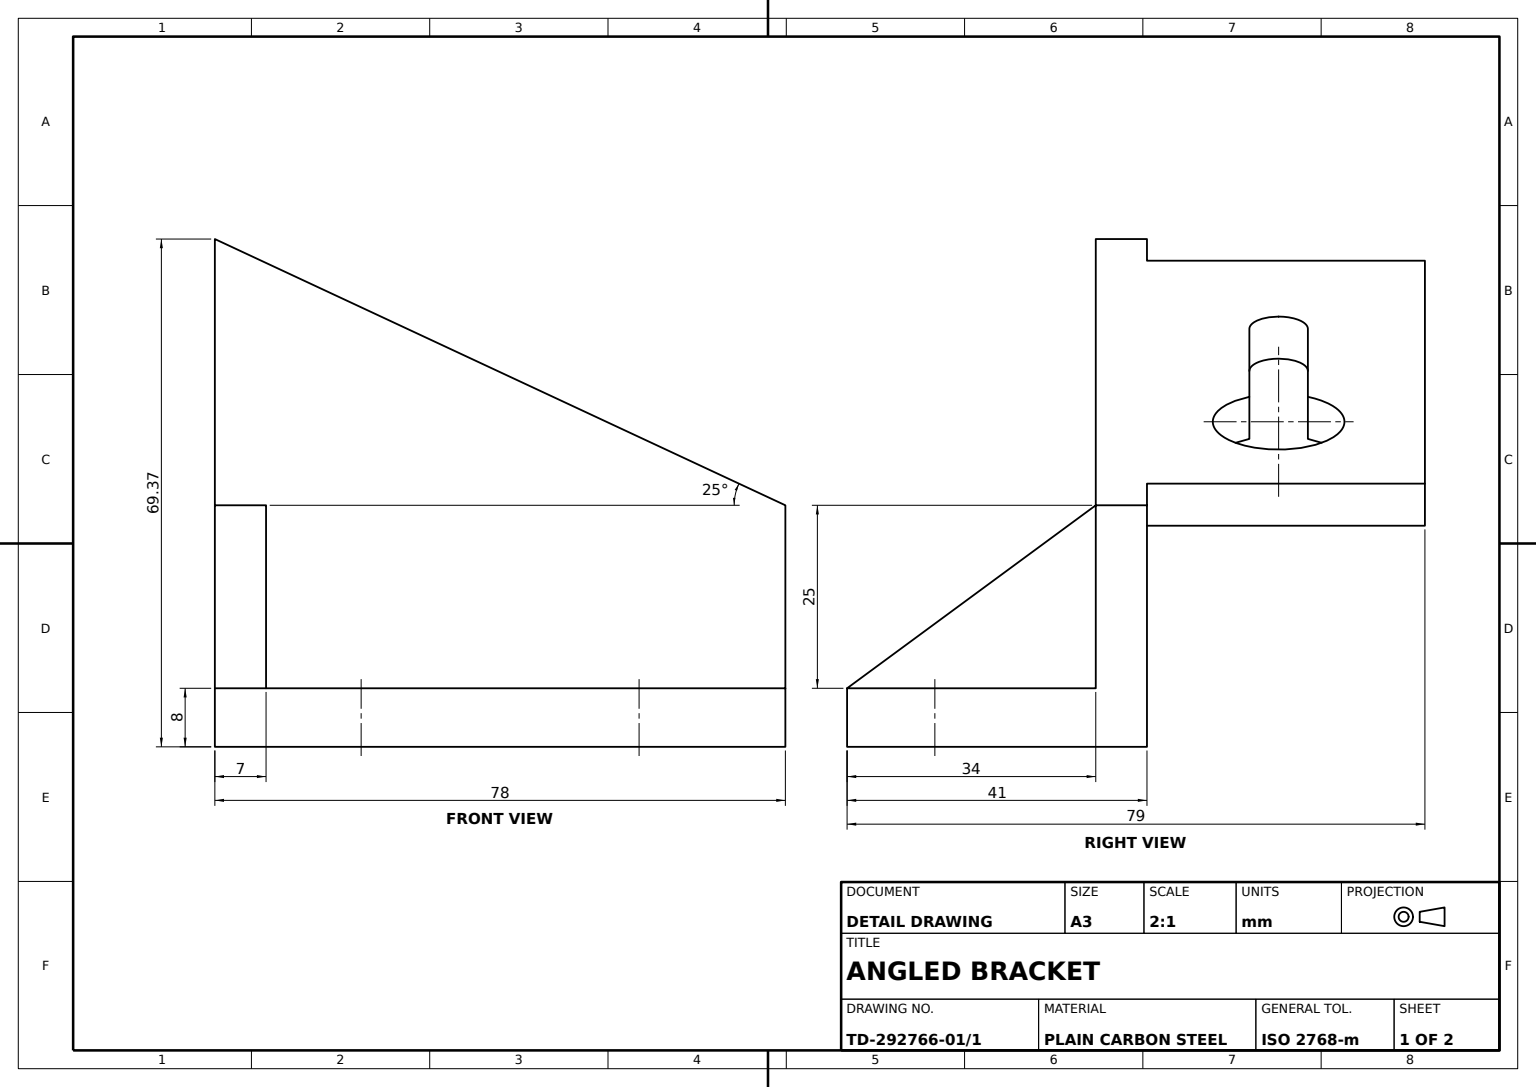
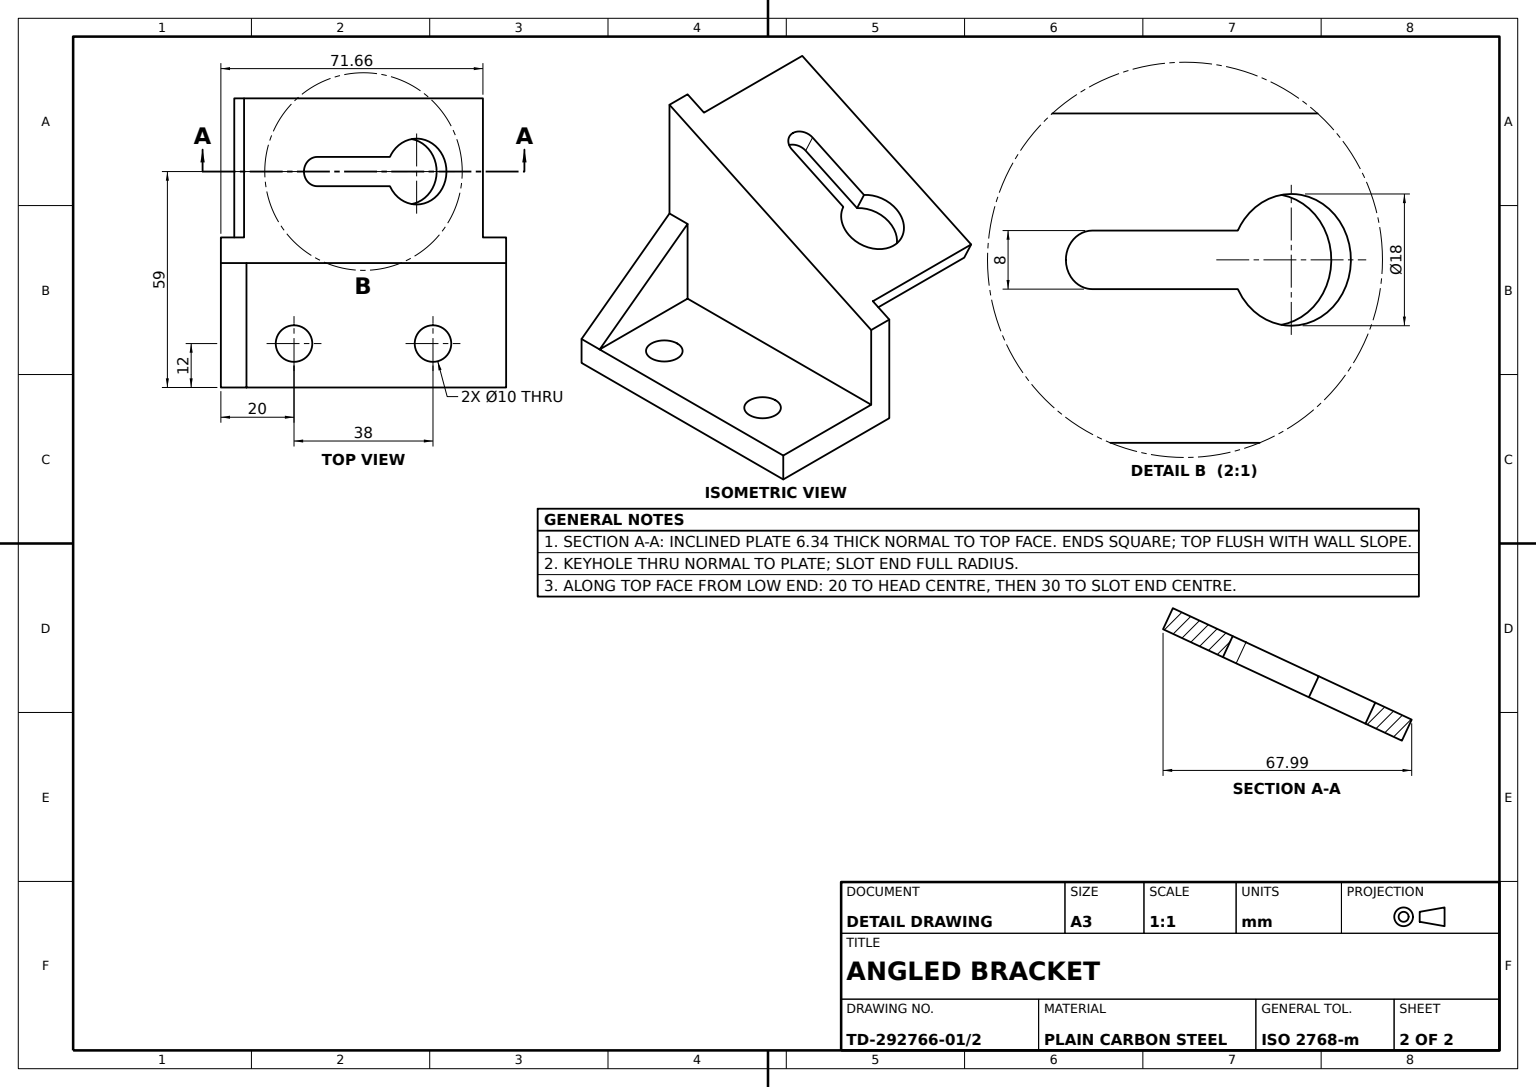
SolidWorks part; units mm, degrees
material "Plain Carbon Steel"
ref_plane "Front Plane" through (0, 0, 0) normal (0, 0, 1) x (1, 0, 0)
ref_plane "Top Plane" through (0, 0, 0) normal (0, 1, 0) x (1, 0, 0)
ref_plane "Right Plane" through (0, 0, 0) normal (1, 0, 0) x (0, 0, -1)
sketch "Base Plate Sketch" plane through (0, 0, 0) normal (0, 1, 0) x (1, 0, 0)
  line L1 (-39, -24.5) -> (39, -24.5)
  line L2 (-39, -24.5) -> (-39, 16.5)
  line L3 (-39, 16.5) -> (39, 16.5)
  line L4 (39, -24.5) -> (39, 16.5)
  circle A0 centre (-19, -12.5) radius 5
  circle A1 centre (19, -12.5) radius 5
  point P0 (0, 0)
  dimension "D3" = 10
  dimension "D4" = 10
  dimension "D1" = 78
  dimension "D2" = 41
  dimension "D5" = 12
  dimension "D6" = 20
  dimension "D7" = 20
  dimension "D8" = 12
  dimension "D9" = 39
  dimension "D10" = 24.5
extrude "Base Plate with Mounting Holes" add sketch "Base Plate Sketch" along normal blind 8
sketch "Upright Wall Sketch" plane through (0, 8, 0) normal (0, 1, 0) x (1, 0, 0)
  line L0 (-39, -24.5) -> (39, -24.5) construction
  line L1 (-39, 16.5) -> (-32, 16.5)
  line L2 (-39, 16.5) -> (-39, -24.5)
  line L3 (-39, -24.5) -> (-32, -24.5)
  line L4 (-32, 16.5) -> (-32, -24.5)
  dimension "D1" = 7
extrude "Upright Wall" add sketch "Upright Wall Sketch" along normal blind 38 contours L2 L3 L4 L1
sketch "Back Plate Sketch" plane through (0, 8, 0) normal (0, 1, 0) x (1, 0, 0)
  line L0 (39, -24.5) -> (39, 16.5) construction
  line L1 (-39, 16.5) -> (39, 16.5)
  line L2 (-39, 16.5) -> (-39, 9.5)
  line L3 (-39, 9.5) -> (39, 9.5)
  line L4 (39, 16.5) -> (39, 9.5)
  dimension "D1" = 7
extrude "Back Plate" add sketch "Back Plate Sketch" along normal blind 82
sketch "Wall Trim Sketch" plane through (-32, 0, 0) normal (1, 0, 0) x (0, 0, -1)
  line L0 (9.5, 33) -> (-24.5, 8)
  line L1 (9.5, 8) -> (9.5, 46) construction
  line L2 (9.5, 33) -> (9.5, 46)
  line L3 (9.5, 46) -> (-24.5, 46)
  line L4 (-24.5, 46) -> (-24.5, 8)
  dimension "D1" = 25
extrude "Wall Trim Cut" cut sketch "Wall Trim Sketch" against normal blind 58
sketch "Angled Trim Sketch 25deg" plane through (0, 0, -9.5) normal (0, 0, 1) x (1, 0, 0)
  line L0 (-39, 69.372) -> (39, 33)
  line L1 (-39, 90) -> (-39, 33) construction
  line L2 (39, 90) -> (39, 8) construction
  line L3 (39, 33) -> (39, 90)
  line L4 (39, 90) -> (-39, 90)
  line L5 (-39, 90) -> (-39, 69.372)
  line L7 (-39, 0) -> (39, 0) construction
  dimension "D1" = 33
  dimension "D2" = 25
extrude "Angled Trim Cut 25deg" cut sketch "Angled Trim Sketch 25deg" against normal blind 58
sketch "Inclined Flange Sketch" plane through (0, 0, -16.5) normal (0, 0, -1) x (-1, 0, 0)
  line L0 (-39, 33) -> (39, 69.372)
  line L1 (39, 69.372) -> (39, 62.372)
  line L2 (39, 69.372) -> (39, 0) construction
  line L3 (-39, 33) -> (-39, 26)
  line L4 (-39, 33) -> (-39, 0) construction
  line L5 (-39, 26) -> (39, 62.372)
  dimension "D1" = 7
  dimension "D2" = 7
extrude "Inclined Flange" add sketch "Inclined Flange Sketch" along normal blind 38
sketch "Flange Profile Cut Sketch" plane through (19.6054, 42.0439, 0) normal (0.4226, 0.9063, 0) x (0.9063, -0.4226, 0)
  line L4 (14.3996, 16.5) -> (14.3996, 54.5)
  line L5 (-64.6639, 54.5) -> (21.3996, 54.5) construction
  line L7 (-57.6639, 54.5) -> (-57.6639, 16.5)
  line L8 (-57.6639, 16.5) -> (-64.6639, 16.5)
  line L9 (-64.6639, 54.5) -> (-64.6639, 9.5) construction
  line L13 (-57.6639, 54.5) -> (-64.6639, 54.5)
  line L14 (-64.6639, 54.5) -> (-64.6639, 16.5)
  line L15 (14.3996, 54.5) -> (24.3579, 54.5)
  line L16 (24.3579, 54.5) -> (24.3579, 16.5)
  line L17 (24.3579, 16.5) -> (14.3996, 16.5)
  dimension "D1" = 79.0635
  dimension "D3" = 7
extrude "Flange Profile Cut" cut sketch "Flange Profile Cut Sketch" against normal blind 38
sketch "Keyhole Slot Sketch" plane through (19.6054, 42.0439, 0) normal (0.4226, 0.9063, 0) x (0.9063, -0.4226, 0)
  line L0 (-35.6004, 38.5) -> (-13.6627, 38.5)
  line L1 (-35.6004, 30.5) -> (-13.6627, 30.5)
  line L2 (14.3996, 54.5) -> (14.3996, 16.5) construction
  line L3 (-57.6639, 54.5) -> (14.3996, 54.5) construction
  arc A0 (-35.6004, 38.5) -> (-35.6004, 30.5) centre (-35.6004, 34.5) ccw
  arc A1 (-13.6627, 30.5) -> (-13.6627, 38.5) centre (-5.6004, 34.5) ccw
  dimension "D1" = 8
  dimension "D2" = 18
  dimension "D3" = 30
  dimension "D4" = 20
  dimension "D5" = 20
extrude "Keyhole Slot Dia18 x W8" cut sketch "Keyhole Slot Sketch" against normal up to next
